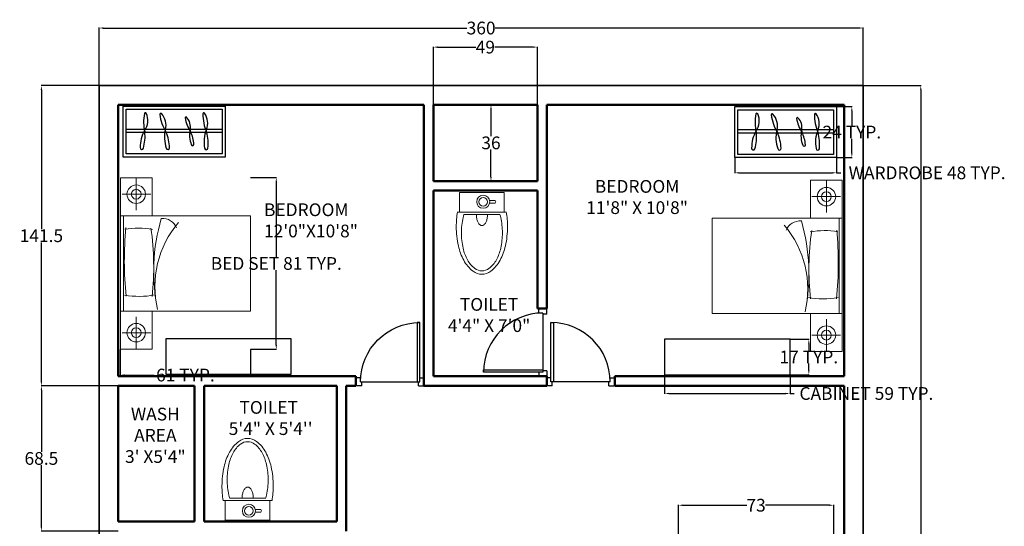
# Model space of a CAD drawing. Units: inches. Extents: x -20 to 10156, y 488 to 2970.
# Tile 5 of 6: x -20 to 444, y 851 to 1090. Entities that reach past the tile are written whole.
import ezdxf

# ---------------------------------------------------------------- set-up
doc = ezdxf.new("R2010")
doc.units = ezdxf.units.IN
doc.header["$MEASUREMENT"] = 0
for name, color, linetype, lineweight in [('A-ANNO-DIMS', 2, 'Continuous', 18), ('A-AREA-IDEN', 7, 'Continuous', 25), ('A-DOOR', 4, 'Continuous', 25), ('A-FLOR-CASE', 8, 'Continuous', 25), ('A-FLOR-FIXT', 9, 'Continuous', 18), ('A-FURN', 8, 'Continuous', 18), ('A-WALL', 7, 'Continuous', 50), ('C-PROP', 7, 'Continuous', 35)]:
    doc.layers.add(name, color=color, linetype=linetype, lineweight=lineweight)
doc.styles.get("Standard").update_dxf_attribs({"font": 'arial.ttf'})
doc.dimstyles.get("Standard").update_dxf_attribs({"dimtxt": 6, "dimasz": 2, "dimexe": 0.18, "dimexo": 0.0625, "dimgap": 0.09, "dimtad": 0, "dimtih": 1, "dimtoh": 1, "dimdec": 0, "dimzin": 0, "dimdsep": 46, "dimlunit": 4, "dimtxsty": 'Standard', "dimcen": 0.09, "dimadec": 0, "dimazin": 0, "dimtfac": 1, "dimtdec": 0, "dimtofl": 0, "dimtmove": 0, "dimatfit": 3, "dimfxl": 1, "dimtolj": 1, "dimtzin": 0, "dimarcsym": 0})

# ---------------------------------------------------------------- blocks, each defined once
blk = doc.blocks.new('A$C7FD35E1A')
for p, q in [((0.0233, 0.5799), (0.0233, 0.4408)), ((0.0233, 0.5799), (0.338, 0.5799)), ((0.338, 0.5799), (0.338, 0.4408)), ((0.2356, 0.5044), (0.275, 0.5044)), ((0.2357, 0.5217), (0.2745, 0.5217)), ((0.3542, 0.4408), (0.0087, 0.4408)), ((0.3093, 0.4224), (0.0536, 0.4224))]:
    blk.add_line(p, q)
for radius in [0.046, 0.0305]:
    blk.add_circle((0.1904, 0.5132), radius)
for centre, radius, start, end in [((0.2685, 0.5129), 0.0107, 307.48803, 55.39402), ((0.6238, 0.337), 0.6238, 170.41844, 180), ((0.3603, 0.3321), 0.3197, 163.59544, 167.42665), ((0.277, 0.4171), 0.1337, 177.71327, 180), ((0.0869, 0.4171), 0.1337, 360, 2.28673), ((0.0026, 0.3321), 0.3197, 12.57335, 16.40456), ((-0.261, 0.337), 0.6238, 0, 9.58156), ((0.5354, 0.2931), 0.4991, 167.42665, 180), ((0.277, 0.4171), 0.1337, 180, 192.53987), ((0.23, 0.4066), 0.0855, 192.53987, 208.23495), ((0.2004, 0.3907), 0.052, 208.23495, 232.35431), ((0.182, 0.3668), 0.0218, 232.35431, 270), ((0.182, 0.3668), 0.0218, 270, 307.64569), ((0.1635, 0.3907), 0.052, 307.64569, 331.76505), ((0.1339, 0.4066), 0.0855, 331.76505, 347.46013), ((0.0869, 0.4171), 0.1337, 347.46013, 0), ((-0.1725, 0.2931), 0.4991, 0, 12.57335), ((0.6238, 0.337), 0.6238, 180, 192.57335), ((0.5354, 0.2931), 0.4991, 180, 192.57335), ((-0.1725, 0.2931), 0.4991, 347.42665, 0), ((-0.261, 0.337), 0.6238, 347.42665, 0), ((0.405, 0.2881), 0.3996, 192.57335, 208.30076), ((0.3603, 0.254), 0.3197, 192.57335, 208.30076), ((0.0026, 0.254), 0.3197, 331.69924, 347.42665), ((-0.0421, 0.2881), 0.3996, 331.69924, 347.42665), ((0.2672, 0.214), 0.2432, 208.30076, 232.43058), ((0.2501, 0.1947), 0.1945, 208.30076, 232.43058), ((0.1128, 0.1947), 0.1945, 307.56942, 331.69924), ((0.0957, 0.214), 0.2432, 307.56942, 331.69924), ((0.1814, 0.1024), 0.1024, 232.43058, 270), ((0.1814, 0.1055), 0.082, 232.43058, 270), ((0.1814, 0.1055), 0.082, 270, 307.56942), ((0.1814, 0.1024), 0.1024, 270, 307.56942)]:
    blk.add_arc(centre, radius, start, end)
blk = doc.blocks.new('A$C041817D3')
for p, q in [((0, 0), (0, 500)), ((0, 500), (1000, 500)), ((1000, 500), (1000, 0)), ((30, 30), (30, 470)), ((30, 470), (970, 470)), ((970, 470), (970, 30)), ((206.7, 270.8), (29.8, 270.8)), ((199, 240.8), (29.8, 240.8)), ((408.8, 240.8), (212.6, 240.8)), ((405.5, 270.8), (216.1, 270.8)), ((647.4, 270.8), (415.1, 270.8)), ((652.4, 240.8), (422, 240.8)), ((807.7, 270.8), (657.5, 270.8)), ((806.2, 240.8), (664.7, 240.8)), ((970.2, 270.8), (817, 270.8)), ((970.2, 240.8), (819.2, 240.8)), ((970, 30), (30, 30)), ((1000, 0), (0, 0))]:
    blk.add_line(p, q)
for centre, radius, start, end in [((621.4, 345.7), 421.4, 168.77299, 193.85802), ((217.3, 425.9), 9.38, 24.60956, 168.77299), ((72.1, 359.4), 169.1, 323.97798, 24.60956), ((368.6, 419.8), 9.38, 42.60956, 186.77299), ((777.7, 468.4), 421.4, 186.77299, 211.85802), ((251, 311.7), 169.1, 345.54145, 42.60956), ((615.5, 385.7), 7.5, 44.60956, 188.77299), ((524.6, 295.9), 135.3, 347.54145, 44.60956), ((791.5, 424.4), 9.38, 34.60956, 178.77299), ((1203.4, 415.6), 421.4, 178.77299, 203.85802), ((660.1, 333.7), 169.1, 337.54145, 34.60956), ((941.3, 435.9), 337.1, 188.77299, 213.85802), ((476.4, 102.2), 310, 149.58385, 181.67451), ((-230.1, 204), 444.3, 344.57561, 5.26247), ((715, 192.1), 310, 165.54145, 199.67451), ((11.6, 70.6), 444.3, 2.57561, 23.26247), ((898.8, 213.2), 248, 167.54145, 201.67451), ((339.9, 96.4), 355.4, 4.57561, 25.26247), ((1102.9, 150.7), 310, 157.54145, 191.67451), ((389.5, 128.2), 444.3, 354.57561, 15.26247), ((681.2, 123.8), 13, 189.40186, 4.57561), ((182.5, 90.2), 16.3, 169.40186, 344.57561), ((439.2, 89.8), 16.3, 187.40186, 2.57561), ((815.5, 87.8), 16.3, 179.40186, 354.57561)]:
    blk.add_arc(centre, radius, start, end)
blk = doc.blocks.new('A$C72DF01B0')
for p, q in [((50, 100), (0, 100)), ((65, 0), (65, 50)), ((780, 50), (80, 50)), ((765, 0), (765, 50)), ((780, 50), (780, 100)), ((780, 100), (830, 100)), ((65, 0), (0, 0)), ((765, 0), (830, 0))]:
    blk.add_line(p, q)
blk.add_lwpolyline([(50, 780), (80, 780), (80, 50), (50, 50)], close=True)
blk.add_arc((50, 50), 730, 0, 90)
blk = doc.blocks.new('BED-WITH-NIGHTSTANDS')
for p, q in [((0, 80.86), (14.96, 80.86)), ((0, 62.91), (0, 80.86)), ((7.48, 73.12), (7.48, 80.95)), ((14.96, 80.86), (14.96, 62.91)), ((7.48, 73.12), (0.91, 73.12)), ((7.48, 73.12), (7.48, 65.64)), ((7.48, 73.12), (14.3, 73.12)), ((0, 62.91), (13.46, 62.91)), ((61.33, 62.91), (0, 62.91)), ((0, 18.04), (0, 62.91)), ((14.96, 62.91), (0, 62.91)), ((1.5, 18.04), (1.5, 62.91)), ((61.33, 18.04), (61.33, 62.91)), ((0, 18.04), (13.46, 18.04)), ((0, 18.04), (13.46, 18.04)), ((61.33, 18.04), (0, 18.04)), ((14.96, 18.04), (0, 18.04)), ((0, 18.04), (0, 0.09)), ((7.48, 7.83), (7.48, 15.31)), ((14.96, 0.09), (14.96, 18.04)), ((7.48, 7.83), (0.91, 7.83)), ((7.48, 7.83), (7.48, 0)), ((7.48, 7.83), (14.3, 7.83)), ((0, 0.09), (14.96, 0.09))]:
    blk.add_line(p, q)
for centre, radius in [((7.48, 73.12), 4.35), ((7.48, 73.12), 2.3), ((7.48, 7.83), 4.35), ((7.48, 7.83), 2.3)]:
    blk.add_circle(centre, radius)
for centre, radius, start, end in [((104.1, 36.77), 88.38, 163.6527, 191.7538), ((19.88, 54.53), 7.14, 22.4412, 94.6731), ((161.95, 41.88), 160.07, 174.4374, 186.047), ((8.44, 20.88), 36.25, 79.3149, 100.0855), ((-111.82, 38.85), 127.54, 353.7104, 8.2351), ((62.88, 29.59), 46.58, 139.6764, 193.4364), ((8.92, 63.63), 38.69, 259.7294, 280.8239)]:
    blk.add_arc(centre, radius, start, end)
blk = doc.blocks.new('BEDROOM-STORAGE-UNIT')
blk.add_lwpolyline([(0, 0), (59.06, 0), (59.06, 16.7), (0, 16.7)], close=True)
blk = doc.blocks.new('*D16')
at = {"layer": 'A-ANNO-DIMS', "color": 0, "lineweight": -2, "transparency": 16777216}
for p, q in [((317.27, 1024.77), (317.27, 1017.45)), ((365.27, 1024.77), (365.27, 1017.45)), ((319.27, 1017.63), (363.27, 1017.63)), ((365.27, 1017.63), (367.27, 1017.63))]:
    blk.add_line(p, q, dxfattribs=at)
at = {"layer": 'A-ANNO-DIMS', "color": 0, "transparency": 16777216}
for points in [[(319.27, 1017.96), (319.27, 1017.29), (317.27, 1017.63)], [(363.27, 1017.96), (363.27, 1017.29), (365.27, 1017.63)]]:
    blk.add_solid(points, dxfattribs=at)
at = {"layer": 'Defpoints', "color": 0, "transparency": 16777216}
for p in [(317.27, 1024.83), (365.27, 1024.83), (365.27, 1017.63)]:
    blk.add_point(p, dxfattribs=at)
at = {"layer": 'A-ANNO-DIMS', "color": 0, "transparency": 16777216, "insert": (407.93, 1017.63), "char_height": 6, "attachment_point": 5}
blk.add_mtext('\\A1;WARDROBE 48 TYP.', dxfattribs=at)
blk = doc.blocks.new('*D17')
at = {"layer": 'A-ANNO-DIMS', "color": 0, "lineweight": -2, "transparency": 16777216}
for p, q in [((365.33, 1048.83), (372.65, 1048.83)), ((372.47, 1046.83), (372.47, 1039.93)), ((372.47, 1026.83), (372.47, 1033.72)), ((365.33, 1024.83), (372.65, 1024.83))]:
    blk.add_line(p, q, dxfattribs=at)
at = {"layer": 'A-ANNO-DIMS', "color": 0, "transparency": 16777216}
for points in [[(372.13, 1046.83), (372.8, 1046.83), (372.47, 1048.83)], [(372.13, 1026.83), (372.8, 1026.83), (372.47, 1024.83)]]:
    blk.add_solid(points, dxfattribs=at)
at = {"layer": 'Defpoints', "color": 0, "transparency": 16777216}
for p in [(365.27, 1048.83), (372.47, 1048.83), (365.27, 1024.83)]:
    blk.add_point(p, dxfattribs=at)
at = {"layer": 'A-ANNO-DIMS', "color": 0, "transparency": 16777216, "insert": (372.47, 1036.83), "char_height": 6, "attachment_point": 5}
blk.add_mtext('\\A1;24 TYP.', dxfattribs=at)
blk = doc.blocks.new('*D18')
at = {"layer": 'A-ANNO-DIMS', "color": 0, "lineweight": -2, "transparency": 16777216}
for p, q in [((89.22, 1015.38), (101.48, 1015.38)), ((101.3, 1013.38), (101.3, 978.09)), ((101.3, 936.43), (101.3, 971.71)), ((89.22, 934.43), (101.48, 934.43))]:
    blk.add_line(p, q, dxfattribs=at)
at = {"layer": 'A-ANNO-DIMS', "color": 0, "transparency": 16777216}
for points in [[(100.97, 1013.38), (101.64, 1013.38), (101.3, 1015.38)], [(100.97, 936.43), (101.64, 936.43), (101.3, 934.43)]]:
    blk.add_solid(points, dxfattribs=at)
at = {"layer": 'Defpoints', "color": 0, "transparency": 16777216}
for p in [(89.16, 1015.38), (101.3, 1015.38), (89.16, 934.43)]:
    blk.add_point(p, dxfattribs=at)
at = {"layer": 'A-ANNO-DIMS', "color": 0, "transparency": 16777216, "insert": (101.3, 974.9), "char_height": 6, "attachment_point": 5}
blk.add_mtext('\\A1;BED SET 81 TYP.', dxfattribs=at)
blk = doc.blocks.new('*D19')
at = {"layer": 'A-ANNO-DIMS', "color": 0, "lineweight": -2, "transparency": 16777216}
for p, q in [((27.83, 934.36), (27.83, 922.1)), ((89.16, 934.36), (89.16, 922.1)), ((29.83, 922.28), (43.79, 922.28)), ((87.16, 922.28), (73.21, 922.28))]:
    blk.add_line(p, q, dxfattribs=at)
at = {"layer": 'A-ANNO-DIMS', "color": 0, "transparency": 16777216}
for points in [[(29.83, 922.62), (29.83, 921.95), (27.83, 922.28)], [(87.16, 922.62), (87.16, 921.95), (89.16, 922.28)]]:
    blk.add_solid(points, dxfattribs=at)
at = {"layer": 'Defpoints', "color": 0, "transparency": 16777216}
for p in [(27.83, 934.43), (89.16, 934.43), (89.16, 922.28)]:
    blk.add_point(p, dxfattribs=at)
at = {"layer": 'A-ANNO-DIMS', "color": 0, "transparency": 16777216, "insert": (58.5, 922.28), "char_height": 6, "attachment_point": 5}
blk.add_mtext('\\A1;61 TYP.', dxfattribs=at)
blk = doc.blocks.new('*D20')
at = {"layer": 'A-ANNO-DIMS', "color": 0, "lineweight": -2, "transparency": 16777216}
for p, q in [((284.27, 922.39), (284.27, 913.42)), ((343.34, 922.39), (343.34, 913.42)), ((286.27, 913.6), (341.34, 913.6)), ((343.34, 913.6), (345.34, 913.6))]:
    blk.add_line(p, q, dxfattribs=at)
at = {"layer": 'A-ANNO-DIMS', "color": 0, "transparency": 16777216}
for points in [[(286.27, 913.93), (286.27, 913.26), (284.27, 913.6)], [(341.34, 913.93), (341.34, 913.26), (343.34, 913.6)]]:
    blk.add_solid(points, dxfattribs=at)
at = {"layer": 'Defpoints', "color": 0, "transparency": 16777216}
for p in [(284.27, 922.46), (343.34, 922.46), (343.34, 913.6)]:
    blk.add_point(p, dxfattribs=at)
at = {"layer": 'A-ANNO-DIMS', "color": 0, "transparency": 16777216, "insert": (379.32, 913.6), "char_height": 6, "attachment_point": 5}
blk.add_mtext('\\A1;CABINET 59 TYP.', dxfattribs=at)
blk = doc.blocks.new('*D21')
at = {"layer": 'A-ANNO-DIMS', "color": 0, "lineweight": -2, "transparency": 16777216}
for p, q in [((343.4, 939.15), (352.38, 939.15)), ((352.2, 937.15), (352.2, 933.91)), ((352.2, 924.46), (352.2, 927.7)), ((343.4, 922.46), (352.38, 922.46))]:
    blk.add_line(p, q, dxfattribs=at)
at = {"layer": 'A-ANNO-DIMS', "color": 0, "transparency": 16777216}
for points in [[(351.86, 937.15), (352.53, 937.15), (352.2, 939.15)], [(351.86, 924.46), (352.53, 924.46), (352.2, 922.46)]]:
    blk.add_solid(points, dxfattribs=at)
at = {"layer": 'Defpoints', "color": 0, "transparency": 16777216}
for p in [(343.34, 939.15), (352.2, 939.15), (343.34, 922.46)]:
    blk.add_point(p, dxfattribs=at)
at = {"layer": 'A-ANNO-DIMS', "color": 0, "transparency": 16777216, "insert": (352.2, 930.8), "char_height": 6, "attachment_point": 5}
blk.add_mtext('\\A1;17 TYP.', dxfattribs=at)
blk = doc.blocks.new('*D23')
at = {"layer": 'A-ANNO-DIMS', "color": 0, "lineweight": -2, "transparency": 16777216}
for p, q in [((290.79, 844.02), (290.79, 861.1)), ((292.79, 860.92), (322.98, 860.92)), ((361.91, 860.92), (331.71, 860.92)), ((363.91, 844.02), (363.91, 861.1))]:
    blk.add_line(p, q, dxfattribs=at)
at = {"layer": 'A-ANNO-DIMS', "color": 0, "transparency": 16777216}
for points in [[(292.79, 861.25), (292.79, 860.58), (290.79, 860.92)], [(361.91, 861.25), (361.91, 860.58), (363.91, 860.92)]]:
    blk.add_solid(points, dxfattribs=at)
at = {"layer": 'Defpoints', "color": 0, "transparency": 16777216}
for p in [(363.91, 860.92), (290.79, 843.96), (363.91, 843.96)]:
    blk.add_point(p, dxfattribs=at)
at = {"layer": 'A-ANNO-DIMS', "color": 0, "transparency": 16777216, "insert": (327.35, 860.92), "char_height": 6, "attachment_point": 5}
blk.add_mtext('\\A1;73', dxfattribs=at)
blk = doc.blocks.new('*D28')
at = {"layer": 'A-ANNO-DIMS', "color": 0, "lineweight": -2, "transparency": 16777216}
for p, q in [((17.8, 1058.79), (17.8, 1086.06)), ((19.8, 1085.88), (191.09, 1085.88)), ((375.8, 1085.88), (204.5, 1085.88)), ((377.8, 1058.79), (377.8, 1086.06))]:
    blk.add_line(p, q, dxfattribs=at)
at = {"layer": 'A-ANNO-DIMS', "color": 0, "transparency": 16777216}
for points in [[(19.8, 1086.21), (19.8, 1085.55), (17.8, 1085.88)], [(375.8, 1086.21), (375.8, 1085.55), (377.8, 1085.88)]]:
    blk.add_solid(points, dxfattribs=at)
at = {"layer": 'Defpoints', "color": 0, "transparency": 16777216}
for p in [(377.8, 1085.88), (17.8, 1058.73), (377.8, 1058.73)]:
    blk.add_point(p, dxfattribs=at)
at = {"layer": 'A-ANNO-DIMS', "color": 0, "transparency": 16777216, "insert": (197.8, 1085.88), "char_height": 6, "attachment_point": 5}
blk.add_mtext('\\A1;360', dxfattribs=at)
blk = doc.blocks.new('*D29')
at = {"layer": 'A-ANNO-DIMS', "color": 0, "lineweight": -2, "transparency": 16777216}
for p, q in [((377.86, 1058.73), (405.13, 1058.73)), ((404.95, 1056.73), (404.95, 791.88)), ((404.95, 520.73), (404.95, 785.58)), ((377.86, 518.73), (405.13, 518.73))]:
    blk.add_line(p, q, dxfattribs=at)
at = {"layer": 'A-ANNO-DIMS', "color": 0, "transparency": 16777216}
for points in [[(404.62, 1056.73), (405.28, 1056.73), (404.95, 1058.73)], [(404.62, 520.73), (405.28, 520.73), (404.95, 518.73)]]:
    blk.add_solid(points, dxfattribs=at)
at = {"layer": 'Defpoints', "color": 0, "transparency": 16777216}
for p in [(377.8, 1058.73), (404.95, 1058.73), (377.8, 518.73)]:
    blk.add_point(p, dxfattribs=at)
at = {"layer": 'A-ANNO-DIMS', "color": 0, "transparency": 16777216, "insert": (404.95, 788.73), "char_height": 6, "attachment_point": 5}
blk.add_mtext('\\A1;540', dxfattribs=at)
blk = doc.blocks.new('*D30')
at = {"layer": 'A-ANNO-DIMS', "color": 0, "lineweight": -2, "transparency": 16777216}
for p, q in [((175.3, 1049.79), (175.3, 1077.06)), ((177.3, 1076.88), (195.28, 1076.88)), ((222.3, 1076.88), (204.31, 1076.88)), ((224.3, 1049.79), (224.3, 1077.06))]:
    blk.add_line(p, q, dxfattribs=at)
at = {"layer": 'A-ANNO-DIMS', "color": 0, "transparency": 16777216}
for points in [[(177.3, 1077.21), (177.3, 1076.55), (175.3, 1076.88)], [(222.3, 1077.21), (222.3, 1076.55), (224.3, 1076.88)]]:
    blk.add_solid(points, dxfattribs=at)
at = {"layer": 'Defpoints', "color": 0, "transparency": 16777216}
for p in [(224.3, 1076.88), (175.3, 1049.73), (224.3, 1049.73)]:
    blk.add_point(p, dxfattribs=at)
at = {"layer": 'A-ANNO-DIMS', "color": 0, "transparency": 16777216, "insert": (199.8, 1076.88), "char_height": 6, "attachment_point": 5}
blk.add_mtext('\\A1;49', dxfattribs=at)
blk = doc.blocks.new('*D31')
at = {"layer": 'A-ANNO-DIMS', "color": 0, "lineweight": -2, "transparency": 16777216}
for p, q in [((17.74, 1058.73), (-9.53, 1058.73)), ((-9.35, 1056.73), (-9.35, 991.13)), ((-9.35, 919.23), (-9.35, 984.83)), ((26.74, 917.23), (-9.53, 917.23))]:
    blk.add_line(p, q, dxfattribs=at)
at = {"layer": 'A-ANNO-DIMS', "color": 0, "transparency": 16777216}
for points in [[(-9.68, 1056.73), (-9.02, 1056.73), (-9.35, 1058.73)], [(-9.68, 919.23), (-9.02, 919.23), (-9.35, 917.23)]]:
    blk.add_solid(points, dxfattribs=at)
at = {"layer": 'Defpoints', "color": 0, "transparency": 16777216}
for p in [(17.8, 1058.73), (-9.35, 917.23), (26.8, 917.23)]:
    blk.add_point(p, dxfattribs=at)
at = {"layer": 'A-ANNO-DIMS', "color": 0, "transparency": 16777216, "insert": (-9.35, 987.98), "char_height": 6, "attachment_point": 5}
blk.add_mtext('\\A1;141.5', dxfattribs=at)
blk = doc.blocks.new('*D32')
at = {"layer": 'A-ANNO-DIMS', "color": 0, "lineweight": -2, "transparency": 16777216}
for p, q in [((26.74, 917.23), (-9.53, 917.23)), ((-9.35, 915.23), (-9.35, 886.13)), ((-9.35, 850.73), (-9.35, 879.83)), ((26.74, 848.73), (-9.53, 848.73))]:
    blk.add_line(p, q, dxfattribs=at)
at = {"layer": 'A-ANNO-DIMS', "color": 0, "transparency": 16777216}
for points in [[(-9.68, 915.23), (-9.02, 915.23), (-9.35, 917.23)], [(-9.68, 850.73), (-9.02, 850.73), (-9.35, 848.73)]]:
    blk.add_solid(points, dxfattribs=at)
at = {"layer": 'Defpoints', "color": 0, "transparency": 16777216}
for p in [(26.8, 917.23), (-9.35, 848.73), (26.8, 848.73)]:
    blk.add_point(p, dxfattribs=at)
at = {"layer": 'A-ANNO-DIMS', "color": 0, "transparency": 16777216, "insert": (-9.35, 882.98), "char_height": 6, "attachment_point": 5}
blk.add_mtext('\\A1;68.5', dxfattribs=at)
blk = doc.blocks.new('*D43')
at = {"layer": 'A-ANNO-DIMS', "color": 0, "lineweight": -2, "transparency": 16777216}
for p, q in [((175.36, 1049.73), (202.63, 1049.73)), ((202.45, 1047.73), (202.45, 1034.89)), ((202.45, 1015.73), (202.45, 1028.57)), ((175.36, 1013.73), (202.63, 1013.73))]:
    blk.add_line(p, q, dxfattribs=at)
at = {"layer": 'A-ANNO-DIMS', "color": 0, "transparency": 16777216}
for points in [[(202.12, 1047.73), (202.78, 1047.73), (202.45, 1049.73)], [(202.12, 1015.73), (202.78, 1015.73), (202.45, 1013.73)]]:
    blk.add_solid(points, dxfattribs=at)
at = {"layer": 'Defpoints', "color": 0, "transparency": 16777216}
for p in [(175.3, 1049.73), (175.3, 1013.73), (202.45, 1013.73)]:
    blk.add_point(p, dxfattribs=at)
at = {"layer": 'A-ANNO-DIMS', "color": 0, "transparency": 16777216, "insert": (202.45, 1031.73), "char_height": 6, "attachment_point": 5}
blk.add_mtext('\\A1;36', dxfattribs=at)

msp = doc.modelspace()

# ---------------------------------------------------------------- linework, layer by layer
at = {"layer": 'A-WALL'}
for p, q in [((26.8, 1049.73), (170.8, 1049.73)), ((26.8, 921.73), (26.8, 1049.73)), ((170.8, 1049.73), (170.8, 917.23)), ((175.3, 1049.73), (224.3, 1049.73)), ((175.3, 1013.73), (175.3, 1049.73)), ((224.3, 1049.73), (224.3, 1013.73)), ((228.8, 1049.73), (228.8, 953.73)), ((228.8, 1049.73), (368.8, 1049.73)), ((368.8, 1049.73), (368.8, 921.73)), ((175.3, 1013.73), (224.3, 1013.73)), ((175.3, 1009.23), (224.3, 1009.23)), ((175.3, 921.73), (175.3, 1009.23)), ((224.3, 1009.23), (224.3, 953.73)), ((224.3, 953.73), (228.8, 953.73)), ((26.8, 921.73), (138.8, 921.73)), ((138.8, 921.73), (138.8, 917.23)), ((175.3, 921.73), (228.8, 921.73)), ((228.8, 921.73), (228.8, 917.23)), ((260.8, 921.73), (368.8, 921.73)), ((260.8, 921.73), (260.8, 917.23)), ((26.8, 917.23), (62.8, 917.23)), ((26.8, 853.23), (26.8, 917.23)), ((62.8, 853.23), (62.8, 917.23)), ((67.3, 853.23), (67.3, 917.23)), ((67.3, 917.23), (129.8, 917.23)), ((129.8, 917.23), (129.8, 853.23)), ((134.3, 917.23), (134.3, 848.73)), ((134.3, 917.23), (138.8, 917.23)), ((170.8, 917.23), (228.8, 917.23)), ((224.3, 917.23), (228.8, 917.23)), ((260.8, 917.23), (368.8, 917.23)), ((260.8, 917.23), (368.8, 917.23)), ((368.8, 917.23), (368.8, 728.73)), ((26.8, 853.23), (62.8, 853.23)), ((67.3, 853.23), (129.8, 853.23))]:
    msp.add_line(p, q, dxfattribs=at)
at = {"layer": 'C-PROP'}
for p, q in [((17.8, 1058.73), (377.8, 1058.73)), ((17.8, 518.73), (17.8, 1058.73)), ((377.8, 1058.73), (377.8, 518.73))]:
    msp.add_line(p, q, dxfattribs=at)

# ---------------------------------------------------------------- block references
at = {"layer": 'A-DOOR', "xscale": 0.0382046374882532, "yscale": 0.0382046374882532, "zscale": 0.0382046374882532, "rotation": 90}
msp.add_blockref('A$C72DF01B0', (228.8, 921.73), dxfattribs=at)
at = {"layer": 'A-DOOR', "yscale": 0.0382046374882532, "zscale": 0.0382046374882532}
for p, xscale in [((170.8, 917.23), -0.0382046374882532), ((228.8, 917.23), 0.0382046374882532)]:
    msp.add_blockref('A$C72DF01B0', p, dxfattribs=dict(at, xscale=xscale))
at = {"layer": 'A-FLOR-CASE', "xscale": 0.048, "yscale": 0.048, "zscale": 0.048}
for p in [(29.2, 1025.08), (317.27, 1024.83)]:
    msp.add_blockref('A$C041817D3', p, dxfattribs=at)
at = {"layer": 'A-FLOR-CASE'}
for p in [(49.25, 922.72), (284.27, 922.46)]:
    msp.add_blockref('BEDROOM-STORAGE-UNIT', p, dxfattribs=at)
at = {"layer": 'A-FLOR-FIXT', "xscale": 66.57190006508344, "yscale": 66.57190006508344, "zscale": 66.57190006508344}
msp.add_blockref('A$C7FD35E1A', (186.1, 969.81), dxfattribs=at)
at = {"layer": 'A-FLOR-FIXT', "xscale": -66.57190006508344, "yscale": 66.57190006508344, "zscale": 66.57190006508344, "rotation": 180}
msp.add_blockref('A$C7FD35E1A', (75.72, 892.45), dxfattribs=at)
at = {"layer": 'A-FURN'}
msp.add_blockref('BED-WITH-NIGHTSTANDS', (27.84, 934.43), dxfattribs=at)
at = {"layer": 'A-FURN', "extrusion": (0, 0, -1), "zscale": -1}
msp.add_blockref('BED-WITH-NIGHTSTANDS', (-367.98, 933.27), dxfattribs=at)

# ---------------------------------------------------------------- texts
at = {"layer": 'A-AREA-IDEN', "char_height": 6, "attachment_point": 1}
for s, width, insert in [('\\pxqc;BEDROOM\\P11\'8" X 10\'8"', 73.4967, (234.55, 1014.22)), ('BEDROOM\\P12\'0"X10\'8"', 124.678, (95.53, 1003.21)), ('\\pxqc,t7;TOILET\\P4\'4" X 7\'0"', 72.417, (165.37, 958.6)), ('\\pxqc;TOILET \\P 5\'4" X 5\'4\'\'', 59.4735, (67.99, 910.04)), ('\\pxqc;WASH \\PAREA\\P3\' X5\'4"', 68.5203, (10.07, 906.88))]:
    msp.add_mtext_dynamic_manual_height_columns(s, width=width, gutter_width=30, heights=[0], dxfattribs=dict(at, insert=insert))

# ---------------------------------------------------------------- dimensions: what is measured, and where the dimension line sits
at = {"layer": 'A-ANNO-DIMS'}
for base, p1, p2, picture, middle in [((377.8, 1085.88), (17.8, 1058.73), (377.8, 1058.73), '*D28', (197.8, 1085.88)), ((224.3, 1076.88), (175.3, 1049.73), (224.3, 1049.73), '*D30', (199.8, 1076.88)), ((363.91, 860.92), (290.79, 843.96), (363.91, 843.96), '*D23', (327.35, 860.92))]:
    dim = msp.add_linear_dim(base=base, p1=p1, p2=p2, dimstyle='Standard', override={"dimdec": 0, "dimlfac": 1, "dimrnd": 0, "dimzin": 0, "dimdsep": 46, "dimlunit": 2}, dxfattribs=at)
    dim.commit()
    dim.dimension.update_dxf_attribs({"geometry": picture, "text_midpoint": middle})
for base, p1, p2, angle, override, picture, middle in [((-9.35, 917.23), (17.8, 1058.73), (26.8, 917.23), 90, {"dimdec": 1, "dimlfac": 1, "dimrnd": 0, "dimzin": 0, "dimdsep": 46, "dimlunit": 2}, '*D31', (-9.35, 987.98)), ((404.95, 1058.73), (377.8, 518.73), (377.8, 1058.73), 90, {"dimdec": 0, "dimlfac": 1, "dimrnd": 0, "dimzin": 0, "dimdsep": 46, "dimlunit": 2}, '*D29', (404.95, 788.73)), ((202.45, 1013.73), (175.3, 1049.73), (175.3, 1013.73), 270, {"dimdec": 0, "dimlfac": 1, "dimrnd": 0, "dimzin": 0, "dimdsep": 46, "dimlunit": 2}, '*D43', (202.45, 1031.73)), ((-9.35, 848.73), (26.8, 917.23), (26.8, 848.73), 90, {"dimdec": 1, "dimlfac": 1, "dimrnd": 0, "dimzin": 0, "dimdsep": 46, "dimlunit": 2}, '*D32', (-9.35, 882.98))]:
    dim = msp.add_linear_dim(base=base, p1=p1, p2=p2, angle=angle, dimstyle='Standard', override=override, dxfattribs=at)
    dim.commit()
    dim.dimension.update_dxf_attribs({"geometry": picture, "text_midpoint": middle})
for base, p1, p2, text, picture, middle in [((372.47, 1048.83), (365.27, 1024.83), (365.27, 1048.83), '<> TYP.', '*D17', (372.47, 1036.83)), ((101.3, 1015.38), (89.16, 934.43), (89.16, 1015.38), 'BED SET <> TYP.', '*D18', (101.3, 974.9)), ((352.2, 939.15), (343.34, 922.46), (343.34, 939.15), '<> TYP.', '*D21', (352.2, 930.8))]:
    dim = msp.add_linear_dim(base=base, p1=p1, p2=p2, angle=90, text=text, dimstyle='Standard', override={"dimdec": 0, "dimlfac": 1, "dimrnd": 0, "dimzin": 0, "dimdsep": 46, "dimlunit": 2}, dxfattribs=at)
    dim.commit()
    dim.dimension.update_dxf_attribs({"geometry": picture, "text_midpoint": middle})
for base, p1, p2, text, picture, middle in [((365.27, 1017.63), (317.27, 1024.83), (365.27, 1024.83), 'WARDROBE <> TYP.', '*D16', (407.93, 1017.63)), ((89.16, 922.28), (27.83, 934.43), (89.16, 934.43), '<> TYP.', '*D19', (58.5, 922.28)), ((343.34, 913.6), (284.27, 922.46), (343.34, 922.46), 'CABINET <> TYP.', '*D20', (379.32, 913.6))]:
    dim = msp.add_linear_dim(base=base, p1=p1, p2=p2, text=text, dimstyle='Standard', override={"dimdec": 0, "dimlfac": 1, "dimrnd": 0, "dimzin": 0, "dimdsep": 46, "dimlunit": 2}, dxfattribs=at)
    dim.commit()
    dim.dimension.update_dxf_attribs({"geometry": picture, "text_midpoint": middle})

doc.saveas('drawing.dxf')
